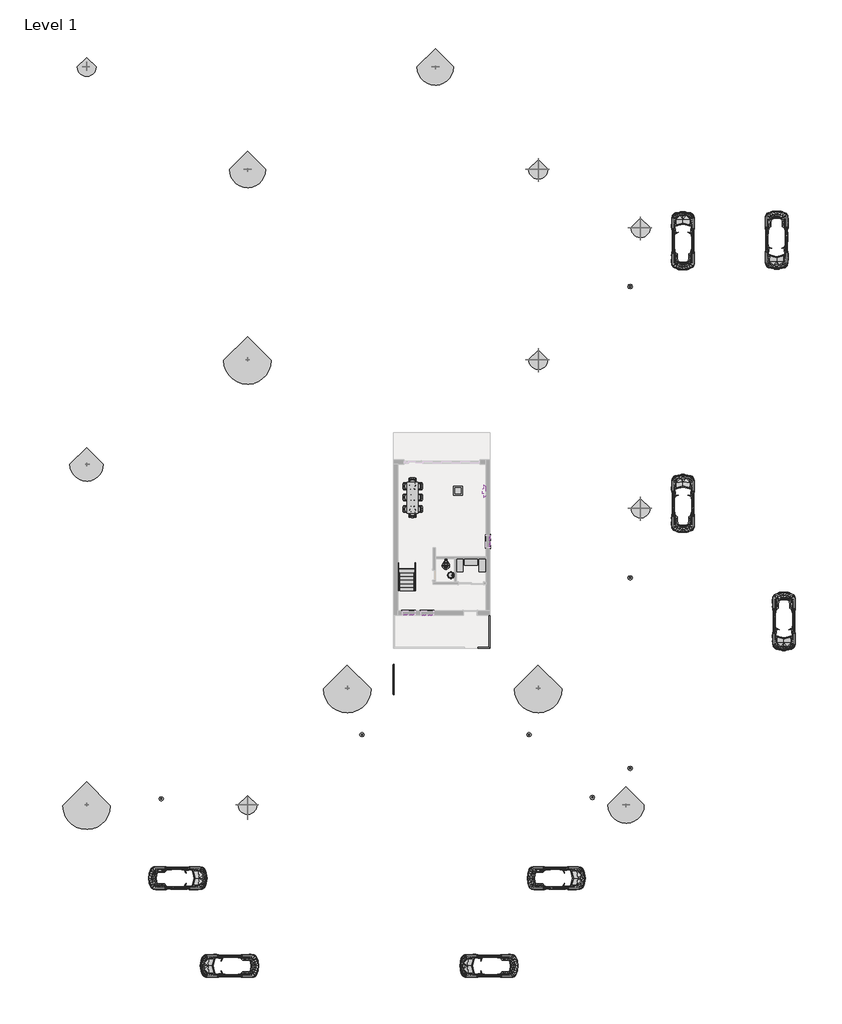
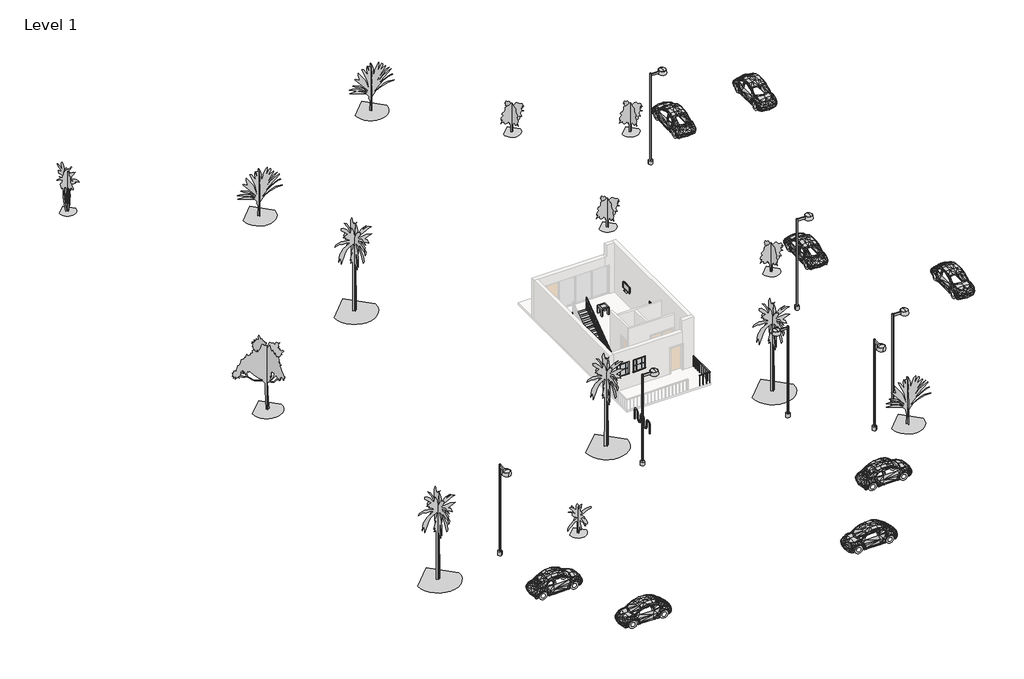
# One storey, part 2 of 2: 21 proxies, 14 furniture elements, 14 geographic elements, 7 light fixtures, 2 flow terminals, 2 members, 2 railings, 1 stair flight.
"""IFC4 building model written with IfcOpenShell, lengths in millimetres."""

from ifc_helpers import new_model, si_unit, frame, origin, origin_with_axes, place, context, project, spatial, polyline, circle_curve, ellipse_curve, outline, extrude, faceted_brep, transform, mapped, element, save
from ifc_brep_helpers import plane_surface, cylinder_surface, advanced_brep
from components import m_bicycle_rack_m_bicycle_rack_69598307, m_muntin_pattern_2x2_m_muntin_pattern_2x2_62480ac4, m_muntin_pattern_2x2_m_muntin_pattern_2x2_4fd78f17, m_rpc_beetle_m_rpc_beetle_aa710b07, m_trim_window_exterior_flat_with_sill_90d3a428, m_trim_window_exterior_flat_with_sill_c06b807c, m_trim_window_interior_flat_picture_frame_6ca9b1f8, m_trim_window_interior_flat_picture_frame_8dc44e6e, m_sink_vanity_round_482_x_482mm_721ec264, m_toilet_commercial_wall_3d_380mm_seat_height_fb359b30, furniture_0810mm_51289c3c, m_furniture_system_storage_cabinet_2_vertical_file_900_x_450_def3fd80, m_seating_auditorium_457_x_610mm_eb3a3c23, m_seating_auditorium_457_x_610mm_4fdbbe14, m_table_coffee_0610_x_0610_x_0610mm_038d1558, m_table_dining_0762_x_2134mm_32ec0f49, m_rpc_tree_tropical_44340318, m_rpc_tree_tropical_0b38fe0e, m_rpc_tree_tropical_cuban_royal_palm_7_5_meters_87faf919, m_rpc_tree_tropical_grass_palm_5_5_meters_0f61173e, m_rpc_tree_tropical_hurricane_palm_3_6_meters_73a83cb7, m_rpc_tree_tropical_japanese_fiber_banana_2_4_meters_2e6d15ad, m_street_light_standard_250w_halogen_277v_204dbcbb, stair_flight_50mm_tread_13mm_riser_6fdf431e

model = new_model("IFC4")

# Units and contexts
model_context = context("Model", 3, world=origin())
ifc_project = project(units=[si_unit("LENGTHUNIT", "METRE", prefix="MILLI")], contexts=[model_context])

# Site, building, storey
site = spatial("IfcSite", under=ifc_project)
building = spatial("IfcBuilding", under=site)
storey = spatial("IfcBuildingStorey", under=building, Name="Level 1", Elevation=0.0)

# Proxies
placement = place(None, origin())
m_bicycle_rack_m_bicycle_rack_shape = m_bicycle_rack_m_bicycle_rack_69598307(model_context)
element("IfcBuildingElementProxy", 1, Name="M_Bicycle Rack : M_Bicycle Rack", ObjectType="M_Bicycle Rack : M_Bicycle Rack", at=placement, inside=storey, context=model_context, shape_type="MappedRepresentation", body=[
    mapped(m_bicycle_rack_m_bicycle_rack_shape, transform((-5369.0317552, -8816.7477501, 0.0), x_axis=(0.0, 1.0, 0.0), y_axis=(-1.0, 0.0, 0.0), z_axis=(0.0, 0.0, 1.0))),
])
m_muntin_pattern_2x2_m_muntin_pattern_2x2_shape = m_muntin_pattern_2x2_m_muntin_pattern_2x2_62480ac4(model_context)
element("IfcBuildingElementProxy", 2, Name="M_Muntin Pattern_2x2 : M_Muntin Pattern_2x2", ObjectType="M_Muntin Pattern_2x2 : M_Muntin Pattern_2x2", at=placement, inside=storey, context=model_context, shape_type="MappedRepresentation", body=[
    mapped(m_muntin_pattern_2x2_m_muntin_pattern_2x2_shape, transform((-4133.1192552, -4407.2227501, 1303.85), x_axis=(-1.0, 0.0, 0.0), y_axis=(0.0, -1.0, 0.0), z_axis=(0.0, 0.0, 1.0))),
])
element("IfcBuildingElementProxy", 3, Name="M_Muntin Pattern_2x2 : M_Muntin Pattern_2x2", ObjectType="M_Muntin Pattern_2x2 : M_Muntin Pattern_2x2", at=placement, inside=storey, context=model_context, shape_type="MappedRepresentation", body=[
    mapped(m_muntin_pattern_2x2_m_muntin_pattern_2x2_shape, transform((-2863.1192552, -4407.2227501, 1303.85), x_axis=(-1.0, 0.0, 0.0), y_axis=(0.0, -1.0, 0.0), z_axis=(0.0, 0.0, 1.0))),
])
element("IfcBuildingElementProxy", 4, Name="M_Muntin Pattern_2x2 : M_Muntin Pattern_2x2", ObjectType="M_Muntin Pattern_2x2 : M_Muntin Pattern_2x2", at=placement, inside=storey, context=model_context, shape_type="MappedRepresentation", body=[
    mapped(m_muntin_pattern_2x2_m_muntin_pattern_2x2_shape, transform((1221.4432448, 819.1647499, 1303.85), x_axis=(0.0, -1.0, 0.0), y_axis=(1.0, 0.0, 0.0), z_axis=(0.0, 0.0, 1.0))),
])
m_muntin_pattern_2x2_m_muntin_pattern_2x2_2_shape = m_muntin_pattern_2x2_m_muntin_pattern_2x2_4fd78f17(model_context)
element("IfcBuildingElementProxy", 5, Name="M_Muntin Pattern_2x2 : M_Muntin Pattern_2x2", ObjectType="M_Muntin Pattern_2x2 : M_Muntin Pattern_2x2", at=placement, inside=storey, context=model_context, shape_type="MappedRepresentation", body=[
    mapped(m_muntin_pattern_2x2_m_muntin_pattern_2x2_2_shape, transform((-4554.9442552, -4407.2227501, 1303.85), x_axis=(1.0, 0.0, 0.0), y_axis=(0.0, 1.0, 0.0), z_axis=(0.0, 0.0, 1.0))),
])
element("IfcBuildingElementProxy", 6, Name="M_Muntin Pattern_2x2 : M_Muntin Pattern_2x2", ObjectType="M_Muntin Pattern_2x2 : M_Muntin Pattern_2x2", at=placement, inside=storey, context=model_context, shape_type="MappedRepresentation", body=[
    mapped(m_muntin_pattern_2x2_m_muntin_pattern_2x2_2_shape, transform((-3284.9442552, -4407.2227501, 1303.85), x_axis=(1.0, 0.0, 0.0), y_axis=(0.0, 1.0, 0.0), z_axis=(0.0, 0.0, 1.0))),
])
element("IfcBuildingElementProxy", 7, Name="M_Muntin Pattern_2x2 : M_Muntin Pattern_2x2", ObjectType="M_Muntin Pattern_2x2 : M_Muntin Pattern_2x2", at=placement, inside=storey, context=model_context, shape_type="MappedRepresentation", body=[
    mapped(m_muntin_pattern_2x2_m_muntin_pattern_2x2_2_shape, transform((1221.4432448, 397.3397499, 1303.85), x_axis=(0.0, 1.0, 0.0), y_axis=(-1.0, 0.0, 0.0), z_axis=(0.0, 0.0, 1.0))),
])
m_rpc_beetle_m_rpc_beetle_shape = m_rpc_beetle_m_rpc_beetle_aa710b07(model_context)
element("IfcBuildingElementProxy", 8, Name="M_RPC Beetle : M_RPC Beetle", ObjectType="M_RPC Beetle : M_RPC Beetle", at=placement, inside=storey, context=model_context, shape_type="MappedRepresentation", body=[
    mapped(m_rpc_beetle_m_rpc_beetle_shape, transform((14420.1682448, 1983.2522499, -152.4), x_axis=(1.0, 0.0, 0.0), y_axis=(0.0, 1.0, 0.0), z_axis=(0.0, 0.0, 1.0))),
])
element("IfcBuildingElementProxy", 9, Name="M_RPC Beetle : M_RPC Beetle", ObjectType="M_RPC Beetle : M_RPC Beetle", at=placement, inside=storey, context=model_context, shape_type="MappedRepresentation", body=[
    mapped(m_rpc_beetle_m_rpc_beetle_shape, transform((21320.1682448, -3616.7477501, -152.4), x_axis=(-1.0, 0.0, 0.0), y_axis=(0.0, -1.0, 0.0), z_axis=(0.0, 0.0, 1.0))),
])
element("IfcBuildingElementProxy", 10, Name="M_RPC Beetle : M_RPC Beetle", ObjectType="M_RPC Beetle : M_RPC Beetle", at=placement, inside=storey, context=model_context, shape_type="MappedRepresentation", body=[
    mapped(m_rpc_beetle_m_rpc_beetle_shape, transform((20820.1682448, 22434.2726811, -152.4), x_axis=(-1.0, 0.0, 0.0), y_axis=(0.0, -1.0, 0.0), z_axis=(0.0, 0.0, 1.0))),
])
element("IfcBuildingElementProxy", 11, Name="M_RPC Beetle : M_RPC Beetle", ObjectType="M_RPC Beetle : M_RPC Beetle", at=placement, inside=storey, context=model_context, shape_type="MappedRepresentation", body=[
    mapped(m_rpc_beetle_m_rpc_beetle_shape, transform((14420.1682448, 19934.2726811, -152.4), x_axis=(1.0, 0.0, 0.0), y_axis=(0.0, 1.0, 0.0), z_axis=(0.0, 0.0, 1.0))),
])
element("IfcBuildingElementProxy", 12, Name="M_RPC Beetle : M_RPC Beetle", ObjectType="M_RPC Beetle : M_RPC Beetle", at=placement, inside=storey, context=model_context, shape_type="MappedRepresentation", body=[
    mapped(m_rpc_beetle_m_rpc_beetle_shape, transform((4520.1682448, -22389.3361723, -152.4), x_axis=(0.0, -1.0, 0.0), y_axis=(1.0, 0.0, 0.0), z_axis=(0.0, 0.0, 1.0))),
])
element("IfcBuildingElementProxy", 13, Name="M_RPC Beetle : M_RPC Beetle", ObjectType="M_RPC Beetle : M_RPC Beetle", at=placement, inside=storey, context=model_context, shape_type="MappedRepresentation", body=[
    mapped(m_rpc_beetle_m_rpc_beetle_shape, transform((2380.1682448, -28389.3361723, -152.4), x_axis=(0.0, 1.0, 0.0), y_axis=(-1.0, 0.0, 0.0), z_axis=(0.0, 0.0, 1.0))),
])
element("IfcBuildingElementProxy", 14, Name="M_RPC Beetle : M_RPC Beetle", ObjectType="M_RPC Beetle : M_RPC Beetle", at=placement, inside=storey, context=model_context, shape_type="MappedRepresentation", body=[
    mapped(m_rpc_beetle_m_rpc_beetle_shape, transform((-15353.4317552, -28389.3361723, -152.4), x_axis=(0.0, 1.0, 0.0), y_axis=(-1.0, 0.0, 0.0), z_axis=(0.0, 0.0, 1.0))),
])
element("IfcBuildingElementProxy", 15, Name="M_RPC Beetle : M_RPC Beetle", ObjectType="M_RPC Beetle : M_RPC Beetle", at=placement, inside=storey, context=model_context, shape_type="MappedRepresentation", body=[
    mapped(m_rpc_beetle_m_rpc_beetle_shape, transform((-21353.4317552, -22389.3361723, -152.4), x_axis=(0.0, -1.0, 0.0), y_axis=(1.0, 0.0, 0.0), z_axis=(0.0, 0.0, 1.0))),
])
m_trim_window_exterior_flat_with_sill_shape = m_trim_window_exterior_flat_with_sill_90d3a428(model_context)
element("IfcBuildingElementProxy", 16, Name="M_Trim-Window-Exterior-Flat : with Sill", ObjectType="M_Trim-Window-Exterior-Flat : with Sill", at=placement, inside=storey, context=model_context, shape_type="MappedRepresentation", body=[
    mapped(m_trim_window_exterior_flat_with_sill_shape, transform((-4344.0317552, -4416.7477501, 2134.0), x_axis=(1.0, 0.0, 0.0), y_axis=(0.0, 0.0, 1.0), z_axis=(0.0, -1.0, 0.0))),
])
element("IfcBuildingElementProxy", 17, Name="M_Trim-Window-Exterior-Flat : with Sill", ObjectType="M_Trim-Window-Exterior-Flat : with Sill", at=placement, inside=storey, context=model_context, shape_type="MappedRepresentation", body=[
    mapped(m_trim_window_exterior_flat_with_sill_shape, transform((-3074.0317552, -4416.7477501, 2134.0), x_axis=(1.0, 0.0, 0.0), y_axis=(0.0, 0.0, 1.0), z_axis=(0.0, -1.0, 0.0))),
])
m_trim_window_exterior_flat_with_sill_2_shape = m_trim_window_exterior_flat_with_sill_c06b807c(model_context)
element("IfcBuildingElementProxy", 18, Name="M_Trim-Window-Exterior-Flat : with Sill", ObjectType="M_Trim-Window-Exterior-Flat : with Sill", at=placement, inside=storey, context=model_context, shape_type="MappedRepresentation", body=[
    mapped(m_trim_window_exterior_flat_with_sill_2_shape, transform((1230.9682448, 608.2522499, 2134.0), x_axis=(0.0, -1.0, 0.0), y_axis=(0.0, 0.0, -1.0), z_axis=(1.0, 0.0, 0.0))),
])
m_trim_window_interior_flat_picture_frame_shape = m_trim_window_interior_flat_picture_frame_6ca9b1f8(model_context)
element("IfcBuildingElementProxy", 19, Name="M_Trim-Window-Interior-Flat : Picture Frame", ObjectType="M_Trim-Window-Interior-Flat : Picture Frame", at=placement, inside=storey, context=model_context, shape_type="MappedRepresentation", body=[
    mapped(m_trim_window_interior_flat_picture_frame_shape, transform((-4344.0317552, -4116.7477501, 2134.0), x_axis=(-1.0, 0.0, 0.0), y_axis=(0.0, 0.0, 1.0), z_axis=(0.0, 1.0, 0.0))),
])
element("IfcBuildingElementProxy", 20, Name="M_Trim-Window-Interior-Flat : Picture Frame", ObjectType="M_Trim-Window-Interior-Flat : Picture Frame", at=placement, inside=storey, context=model_context, shape_type="MappedRepresentation", body=[
    mapped(m_trim_window_interior_flat_picture_frame_shape, transform((-3074.0317552, -4116.7477501, 2134.0), x_axis=(-1.0, 0.0, 0.0), y_axis=(0.0, 0.0, 1.0), z_axis=(0.0, 1.0, 0.0))),
])
m_trim_window_interior_flat_picture_frame_2_shape = m_trim_window_interior_flat_picture_frame_8dc44e6e(model_context)
element("IfcBuildingElementProxy", 21, Name="M_Trim-Window-Interior-Flat : Picture Frame", ObjectType="M_Trim-Window-Interior-Flat : Picture Frame", at=placement, inside=storey, context=model_context, shape_type="MappedRepresentation", body=[
    mapped(m_trim_window_interior_flat_picture_frame_2_shape, transform((930.9682448, 608.2522499, 2134.0), x_axis=(0.0, 1.0, 0.0), y_axis=(0.0, 0.0, -1.0), z_axis=(-1.0, 0.0, 0.0))),
])

# Flow terminals
m_sink_vanity_round_482_x_482mm_shape = m_sink_vanity_round_482_x_482mm_721ec264(model_context)
element("IfcFlowTerminal", 22, ObjectType="M_Sink Vanity-Round : 482 x 482mm", at=placement, inside=storey, context=model_context, shape_type="MappedRepresentation", body=[
    mapped(m_sink_vanity_round_482_x_482mm_shape, transform((-1544.5577535, -1590.0960096, 0.0), x_axis=(0.0, -1.0, 0.0), y_axis=(1.0, 0.0, 0.0), z_axis=(0.0, 0.0, 1.0))),
])
m_toilet_commercial_wall_3d_380mm_seat_height_shape = m_toilet_commercial_wall_3d_380mm_seat_height_fb359b30(model_context)
element("IfcFlowTerminal", 23, ObjectType="M_Toilet-Commercial-Wall-3D : 380mm Seat Height", at=placement, inside=storey, context=model_context, shape_type="MappedRepresentation", body=[
    mapped(m_toilet_commercial_wall_3d_380mm_seat_height_shape, transform((-1388.1286014, -491.7477501, 0.0), x_axis=(-1.0, 0.0, 0.0), y_axis=(0.0, -1.0, 0.0), z_axis=(0.0, 0.0, 1.0))),
])

# Furniture
furniture_0810mm_shape = furniture_0810mm_51289c3c(model_context)
element("IfcFurniture", 24, ObjectType="0810mm", at=placement, inside=storey, context=model_context, shape_type="MappedRepresentation", body=[
    mapped(furniture_0810mm_shape, transform((866.2308395, 4039.3077357, 1219.2), x_axis=(0.0, -1.0, 0.0), y_axis=(1.0, 0.0, 0.0), z_axis=(0.0, 0.0, 1.0))),
])
m_furniture_system_storage_cabinet_2_vertical_file_900_x_450_shape = m_furniture_system_storage_cabinet_2_vertical_file_900_x_450_def3fd80(model_context)
element("IfcFurniture", 25, ObjectType="M_Furniture_System-Storage-Cabinet-2_Vertical_File : 900 x 450 x 650mm", at=placement, inside=storey, context=model_context, shape_type="MappedRepresentation", body=[
    mapped(m_furniture_system_storage_cabinet_2_vertical_file_900_x_450_shape, transform((-619.0317552, -1016.7477501, 0.0), x_axis=(0.0, 1.0, 0.0), y_axis=(-1.0, 0.0, 0.0), z_axis=(0.0, 0.0, 1.0))),
])
element("IfcFurniture", 26, ObjectType="M_Furniture_System-Storage-Cabinet-2_Vertical_File : 900 x 450 x 650mm", at=placement, inside=storey, context=model_context, shape_type="MappedRepresentation", body=[
    mapped(m_furniture_system_storage_cabinet_2_vertical_file_900_x_450_shape, transform((480.9682448, -1016.7477501, 0.0), x_axis=(0.0, -1.0, 0.0), y_axis=(1.0, 0.0, 0.0), z_axis=(0.0, 0.0, 1.0))),
])
element("IfcFurniture", 27, ObjectType="M_Furniture_System-Storage-Cabinet-2_Vertical_File : 900 x 450 x 650mm", at=placement, inside=storey, context=model_context, shape_type="MappedRepresentation", body=[
    mapped(m_furniture_system_storage_cabinet_2_vertical_file_900_x_450_shape, transform((-69.0317552, -1016.7477501, 0.0), x_axis=(1.0, 0.0, 0.0), y_axis=(0.0, 1.0, 0.0), z_axis=(0.0, 0.0, 1.0))),
])
m_seating_auditorium_457_x_610mm_shape = m_seating_auditorium_457_x_610mm_eb3a3c23(model_context)
element("IfcFurniture", 28, ObjectType="M_Seating-Auditorium : 457 x 610mm", at=placement, inside=storey, context=model_context, shape_type="MappedRepresentation", body=[
    mapped(m_seating_auditorium_457_x_610mm_shape, transform((-4639.907165, 4542.5801187, 0.0), x_axis=(0.0, -1.0, 0.0), y_axis=(1.0, 0.0, 0.0), z_axis=(0.0, 0.0, 1.0))),
])
element("IfcFurniture", 29, ObjectType="M_Seating-Auditorium : 457 x 610mm", at=placement, inside=storey, context=model_context, shape_type="MappedRepresentation", body=[
    mapped(m_seating_auditorium_457_x_610mm_shape, transform((-3498.1563454, 4221.124381, 0.0), x_axis=(0.0, 1.0, 0.0), y_axis=(-1.0, 0.0, 0.0), z_axis=(0.0, 0.0, 1.0))),
])
element("IfcFurniture", 30, ObjectType="M_Seating-Auditorium : 457 x 610mm", at=placement, inside=storey, context=model_context, shape_type="MappedRepresentation", body=[
    mapped(m_seating_auditorium_457_x_610mm_shape, transform((-3908.3038863, 4860.1276597, 0.0), x_axis=(-1.0, 0.0, 0.0), y_axis=(0.0, -1.0, 0.0), z_axis=(0.0, 0.0, 1.0))),
])
element("IfcFurniture", 31, ObjectType="M_Seating-Auditorium : 457 x 610mm", at=placement, inside=storey, context=model_context, shape_type="MappedRepresentation", body=[
    mapped(m_seating_auditorium_457_x_610mm_shape, transform((-4229.759624, 2346.37684, 0.0), x_axis=(1.0, 0.0, 0.0), y_axis=(0.0, 1.0, 0.0), z_axis=(0.0, 0.0, 1.0))),
])
m_seating_auditorium_457_x_610mm_2_shape = m_seating_auditorium_457_x_610mm_4fdbbe14(model_context)
element("IfcFurniture", 32, ObjectType="M_Seating-Auditorium : 457 x 610mm", at=placement, inside=storey, context=model_context, shape_type="MappedRepresentation", body=[
    mapped(m_seating_auditorium_457_x_610mm_2_shape, transform((-4639.907165, 2663.924381, 0.0), x_axis=(0.0, 1.0, 0.0), y_axis=(-1.0, 0.0, 0.0), z_axis=(0.0, 0.0, 1.0))),
])
element("IfcFurniture", 33, ObjectType="M_Seating-Auditorium : 457 x 610mm", at=placement, inside=storey, context=model_context, shape_type="MappedRepresentation", body=[
    mapped(m_seating_auditorium_457_x_610mm_2_shape, transform((-3498.1563454, 2985.3801187, 0.0), x_axis=(0.0, -1.0, 0.0), y_axis=(1.0, 0.0, 0.0), z_axis=(0.0, 0.0, 1.0))),
])
element("IfcFurniture", 34, ObjectType="M_Seating-Auditorium : 457 x 610mm", at=placement, inside=storey, context=model_context, shape_type="MappedRepresentation", body=[
    mapped(m_seating_auditorium_457_x_610mm_2_shape, transform((-4639.907165, 3463.924381, 0.0), x_axis=(0.0, 1.0, 0.0), y_axis=(-1.0, 0.0, 0.0), z_axis=(0.0, 0.0, 1.0))),
])
element("IfcFurniture", 35, ObjectType="M_Seating-Auditorium : 457 x 610mm", at=placement, inside=storey, context=model_context, shape_type="MappedRepresentation", body=[
    mapped(m_seating_auditorium_457_x_610mm_2_shape, transform((-3498.1563454, 3785.3801187, 0.0), x_axis=(0.0, -1.0, 0.0), y_axis=(1.0, 0.0, 0.0), z_axis=(0.0, 0.0, 1.0))),
])
m_table_coffee_0610_x_0610_x_0610mm_shape = m_table_coffee_0610_x_0610_x_0610mm_038d1558(model_context)
element("IfcFurniture", 36, ObjectType="M_Table-Coffee : 0610 x 0610 x 0610mm", at=placement, inside=storey, context=model_context, shape_type="MappedRepresentation", body=[
    mapped(m_table_coffee_0610_x_0610_x_0610mm_shape, transform((-997.2975219, 3978.0411721, 0.0), x_axis=(1.0, 0.0, 0.0), y_axis=(0.0, 1.0, 0.0), z_axis=(0.0, 0.0, 1.0))),
])
m_table_dining_0762_x_2134mm_shape = m_table_dining_0762_x_2134mm_32ec0f49(model_context)
element("IfcFurniture", 37, ObjectType="M_Table-Dining : 0762 x 2134mm", at=placement, inside=storey, context=model_context, shape_type="MappedRepresentation", body=[
    mapped(m_table_dining_0762_x_2134mm_shape, transform((-3973.8206774, 3584.9864832, 0.0), x_axis=(0.0, 1.0, 0.0), y_axis=(-1.0, 0.0, 0.0), z_axis=(0.0, 0.0, 1.0))),
])

# Geographic elements
m_rpc_tree_tropical_shape = m_rpc_tree_tropical_44340318(model_context)
element("IfcGeographicElement", 38, ObjectType="M_RPC Tree - Tropical", at=placement, inside=storey, context=model_context, shape_type="MappedRepresentation", body=[
    mapped(m_rpc_tree_tropical_shape, transform((10519.9715737, -17389.3361723, -152.4), x_axis=(1.0, 0.0, 0.0), y_axis=(0.0, 1.0, 0.0), z_axis=(0.0, 0.0, 1.0))),
])
element("IfcGeographicElement", 39, ObjectType="M_RPC Tree - Tropical", at=placement, inside=storey, context=model_context, shape_type="MappedRepresentation", body=[
    mapped(m_rpc_tree_tropical_shape, transform((-2519.2284263, 33034.2726811, -152.4), x_axis=(1.0, 0.0, 0.0), y_axis=(0.0, 1.0, 0.0), z_axis=(0.0, 0.0, 1.0))),
])
element("IfcGeographicElement", 40, ObjectType="M_RPC Tree - Tropical", at=placement, inside=storey, context=model_context, shape_type="MappedRepresentation", body=[
    mapped(m_rpc_tree_tropical_shape, transform((-15353.6284263, 26034.2726811, -152.4), x_axis=(1.0, 0.0, 0.0), y_axis=(0.0, 1.0, 0.0), z_axis=(0.0, 0.0, 1.0))),
])
m_rpc_tree_tropical_2_shape = m_rpc_tree_tropical_0b38fe0e(model_context)
element("IfcGeographicElement", 41, ObjectType="M_RPC Tree - Tropical", at=placement, inside=storey, context=model_context, shape_type="MappedRepresentation", body=[
    mapped(m_rpc_tree_tropical_2_shape, transform((11519.9715737, 2883.2522499, -152.4), x_axis=(1.0, 0.0, 0.0), y_axis=(0.0, 1.0, 0.0), z_axis=(0.0, 0.0, 1.0))),
])
element("IfcGeographicElement", 42, ObjectType="M_RPC Tree - Tropical", at=placement, inside=storey, context=model_context, shape_type="MappedRepresentation", body=[
    mapped(m_rpc_tree_tropical_2_shape, transform((11519.9715737, 22034.2726811, -152.4), x_axis=(1.0, 0.0, 0.0), y_axis=(0.0, 1.0, 0.0), z_axis=(0.0, 0.0, 1.0))),
])
element("IfcGeographicElement", 43, ObjectType="M_RPC Tree - Tropical", at=placement, inside=storey, context=model_context, shape_type="MappedRepresentation", body=[
    mapped(m_rpc_tree_tropical_2_shape, transform((4519.9715737, 26034.2726811, -152.4), x_axis=(1.0, 0.0, 0.0), y_axis=(0.0, 1.0, 0.0), z_axis=(0.0, 0.0, 1.0))),
])
element("IfcGeographicElement", 44, ObjectType="M_RPC Tree - Tropical", at=placement, inside=storey, context=model_context, shape_type="MappedRepresentation", body=[
    mapped(m_rpc_tree_tropical_2_shape, transform((4519.9715737, 13034.2726811, -152.4), x_axis=(1.0, 0.0, 0.0), y_axis=(0.0, 1.0, 0.0), z_axis=(0.0, 0.0, 1.0))),
])
m_rpc_tree_tropical_cuban_royal_palm_7_5_meters_shape = m_rpc_tree_tropical_cuban_royal_palm_7_5_meters_87faf919(model_context)
element("IfcGeographicElement", 45, ObjectType="M_RPC Tree - Tropical : Cuban Royal Palm - 7.5 Meters", at=placement, inside=storey, context=model_context, shape_type="MappedRepresentation", body=[
    mapped(m_rpc_tree_tropical_cuban_royal_palm_7_5_meters_shape, transform((-8529.2284263, -9416.7477501, -152.4), x_axis=(1.0, 0.0, 0.0), y_axis=(0.0, 1.0, 0.0), z_axis=(0.0, 0.0, 1.0))),
])
element("IfcGeographicElement", 46, ObjectType="M_RPC Tree - Tropical : Cuban Royal Palm - 7.5 Meters", at=placement, inside=storey, context=model_context, shape_type="MappedRepresentation", body=[
    mapped(m_rpc_tree_tropical_cuban_royal_palm_7_5_meters_shape, transform((4519.9715737, -9416.7477501, -152.4), x_axis=(1.0, 0.0, 0.0), y_axis=(0.0, 1.0, 0.0), z_axis=(0.0, 0.0, 1.0))),
])
element("IfcGeographicElement", 47, ObjectType="M_RPC Tree - Tropical : Cuban Royal Palm - 7.5 Meters", at=placement, inside=storey, context=model_context, shape_type="MappedRepresentation", body=[
    mapped(m_rpc_tree_tropical_cuban_royal_palm_7_5_meters_shape, transform((-26353.6284263, -17389.3361723, -152.4), x_axis=(1.0, 0.0, 0.0), y_axis=(0.0, 1.0, 0.0), z_axis=(0.0, 0.0, 1.0))),
])
element("IfcGeographicElement", 48, ObjectType="M_RPC Tree - Tropical : Cuban Royal Palm - 7.5 Meters", at=placement, inside=storey, context=model_context, shape_type="MappedRepresentation", body=[
    mapped(m_rpc_tree_tropical_cuban_royal_palm_7_5_meters_shape, transform((-15353.6284263, 13034.2726811, -152.4), x_axis=(1.0, 0.0, 0.0), y_axis=(0.0, 1.0, 0.0), z_axis=(0.0, 0.0, 1.0))),
])
m_rpc_tree_tropical_grass_palm_5_5_meters_shape = m_rpc_tree_tropical_grass_palm_5_5_meters_0f61173e(model_context)
element("IfcGeographicElement", 49, ObjectType="M_RPC Tree - Tropical : Grass Palm - 5.5 Meters", at=placement, inside=storey, context=model_context, shape_type="MappedRepresentation", body=[
    mapped(m_rpc_tree_tropical_grass_palm_5_5_meters_shape, transform((-26353.6284263, 5883.2522499, -152.4), x_axis=(1.0, 0.0, 0.0), y_axis=(0.0, 1.0, 0.0), z_axis=(0.0, 0.0, 1.0))),
])
m_rpc_tree_tropical_hurricane_palm_3_6_meters_shape = m_rpc_tree_tropical_hurricane_palm_3_6_meters_73a83cb7(model_context)
element("IfcGeographicElement", 50, ObjectType="M_RPC Tree - Tropical : Hurricane Palm - 3.6 Meters", at=placement, inside=storey, context=model_context, shape_type="MappedRepresentation", body=[
    mapped(m_rpc_tree_tropical_hurricane_palm_3_6_meters_shape, transform((-26353.6284263, 33034.2726811, -152.4), x_axis=(1.0, 0.0, 0.0), y_axis=(0.0, 1.0, 0.0), z_axis=(0.0, 0.0, 1.0))),
])
m_rpc_tree_tropical_japanese_fiber_banana_2_4_meters_shape = m_rpc_tree_tropical_japanese_fiber_banana_2_4_meters_2e6d15ad(model_context)
element("IfcGeographicElement", 51, ObjectType="M_RPC Tree - Tropical : Japanese Fiber Banana - 2.4 Meters", at=placement, inside=storey, context=model_context, shape_type="MappedRepresentation", body=[
    mapped(m_rpc_tree_tropical_japanese_fiber_banana_2_4_meters_shape, transform((-15353.6284263, -17389.3361723, -152.4), x_axis=(1.0, 0.0, 0.0), y_axis=(0.0, 1.0, 0.0), z_axis=(0.0, 0.0, 1.0))),
])

# Light fixtures
m_street_light_standard_250w_halogen_277v_shape = m_street_light_standard_250w_halogen_277v_204dbcbb(model_context)
element("IfcLightFixture", 52, ObjectType="M_Street Light - Standard", at=placement, inside=storey, context=model_context, shape_type="MappedRepresentation", body=[
    mapped(m_street_light_standard_250w_halogen_277v_shape, transform((-7527.8317552, -12589.3361723, -152.4), x_axis=(-1.0, 0.0, 0.0), y_axis=(0.0, -1.0, 0.0), z_axis=(0.0, 0.0, 1.0))),
])
element("IfcLightFixture", 53, ObjectType="M_Street Light - Standard : 250W Halogen - 277V", at=placement, inside=storey, context=model_context, shape_type="MappedRepresentation", body=[
    mapped(m_street_light_standard_250w_halogen_277v_shape, transform((3894.5682448, -12589.3361723, -152.4), x_axis=(1.0, 0.0, 0.0), y_axis=(0.0, 1.0, 0.0), z_axis=(0.0, 0.0, 1.0))),
])
element("IfcLightFixture", 54, ObjectType="M_Street Light - Standard : 400W Halogen - 120V", at=placement, inside=storey, context=model_context, shape_type="MappedRepresentation", body=[
    mapped(m_street_light_standard_250w_halogen_277v_shape, transform((8220.1682448, -16874.9361723, -152.4), x_axis=(0.0, 1.0, 0.0), y_axis=(-1.0, 0.0, 0.0), z_axis=(0.0, 0.0, 1.0))),
])
element("IfcLightFixture", 55, ObjectType="M_Street Light - Standard : 400W Halogen - 120V", at=placement, inside=storey, context=model_context, shape_type="MappedRepresentation", body=[
    mapped(m_street_light_standard_250w_halogen_277v_shape, transform((10805.7682448, -14889.3361723, -152.4), x_axis=(-1.0, 0.0, 0.0), y_axis=(0.0, -1.0, 0.0), z_axis=(0.0, 0.0, 1.0))),
])
element("IfcLightFixture", 56, ObjectType="M_Street Light - Standard : 400W Halogen - 120V", at=placement, inside=storey, context=model_context, shape_type="MappedRepresentation", body=[
    mapped(m_street_light_standard_250w_halogen_277v_shape, transform((10805.7682448, -1866.7477501, -152.4), x_axis=(-1.0, 0.0, 0.0), y_axis=(0.0, -1.0, 0.0), z_axis=(0.0, 0.0, 1.0))),
])
element("IfcLightFixture", 57, ObjectType="M_Street Light - Standard : 400W Halogen - 120V", at=placement, inside=storey, context=model_context, shape_type="MappedRepresentation", body=[
    mapped(m_street_light_standard_250w_halogen_277v_shape, transform((10805.7682448, 18034.2726811, -152.4), x_axis=(-1.0, 0.0, 0.0), y_axis=(0.0, -1.0, 0.0), z_axis=(0.0, 0.0, 1.0))),
])
element("IfcLightFixture", 58, ObjectType="M_Street Light - Standard : 400W Halogen - 120V", at=placement, inside=storey, context=model_context, shape_type="MappedRepresentation", body=[
    mapped(m_street_light_standard_250w_halogen_277v_shape, transform((-21253.4317552, -16974.9361723, -152.4), x_axis=(0.0, 1.0, 0.0), y_axis=(-1.0, 0.0, 0.0), z_axis=(0.0, 0.0, 1.0))),
])

# Members
element("IfcMember", 59, ObjectType="Stringer - 50mm Width", at=placement, inside=storey, context=model_context, shape_type="SweptSolid", body=[
    extrude(outline(polyline([(-2766.7477501, 0.0), (-2766.7477501, 253.5299646), (1233.2522499, 3265.2946705), (1233.2522499, 2764.5879036), (-2438.4660596, 0.0), (-2766.7477501, 0.0)])), frame((-5069.0317552, 0.0, 0.0), z_axis=(1.0, 0.0, 0.0), x_axis=(0.0, 1.0, 0.0)), (0.0, 0.0, 1.0), 50.0),
])
element("IfcMember", 60, ObjectType="Stringer - 50mm Width", at=placement, inside=storey, context=model_context, shape_type="SweptSolid", body=[
    extrude(outline(polyline([(-2766.7477501, 0.0), (-2766.7477501, 253.5299646), (1233.2522499, 3265.2946705), (1233.2522499, 2764.5879036), (-2438.4660596, 0.0), (-2766.7477501, 0.0)])), frame((-3919.0317552, 0.0, 0.0), z_axis=(1.0, 0.0, 0.0), x_axis=(0.0, 1.0, 0.0)), (0.0, 0.0, 1.0), 50.0),
])

# Railings
element("IfcRailing", 61, ObjectType="900mm Pipe", at=placement, inside=storey, context=model_context, shape_type="AdvancedBrep", body=[
    advanced_brep(
    [(-3924.4317552, -2766.7477501, 1063.1999558), (-3964.4317552, -2766.7477501, 1063.1999558), (-3924.4317552, 1233.2522499, 4074.9646617), (-3964.4317552, 1233.2522499, 4074.9646617)],
    [
        (0, 1, ellipse_curve(frame((-3944.4317552, -2766.7477501, 1063.1999558), z_axis=(0.0, -1.0, 0.0), x_axis=(0.0, 0.0, -1.0)), 25.0353383, 20.0)),
        (1, 0, ellipse_curve(frame((-3944.4317552, -2766.7477501, 1063.1999558), z_axis=(0.0, -1.0, 0.0), x_axis=(0.0, 0.0, -1.0)), 25.0353383, 20.0)),
        (2, 3, ellipse_curve(frame((-3944.4317552, 1233.2522499, 4074.9646617), z_axis=(0.0, 1.0, 0.0), x_axis=(0.0, 0.0, -1.0)), 25.0353383, 20.0)),
        (3, 2, ellipse_curve(frame((-3944.4317552, 1233.2522499, 4074.9646617), z_axis=(0.0, 1.0, 0.0), x_axis=(0.0, 0.0, -1.0)), 25.0353383, 20.0)),
        (0, 2),
        (3, 1),
    ],
    [
        plane_surface(frame((-3944.4317552, -2766.7477501, 1088.2352941), z_axis=(0.0, -1.0, 0.0), x_axis=(0.0, 0.0, 1.0))),
        plane_surface(frame((-3944.4317552, 1233.2522499, 4100.0), z_axis=(0.0, 1.0, 0.0), x_axis=(0.0, 0.0, 1.0))),
        cylinder_surface(frame((-3944.4317552, -2754.7176962, 1072.2578787), z_axis=(0.0, -0.7988707691396074, -0.6015026967639399), x_axis=(-1.0, 0.0, 0.0)), 20.0),
    ],
    [
        (0, [[1, 2]]),
        (1, [[3, 4]]),
        (2, [[-1, 5, -4, 6]]),
        (2, [[-2, -6, -3, -5]]),
    ],
),
    advanced_brep(
    [(-3959.4317552, -2766.7477501, 869.4587904), (-3929.4317552, -2766.7477501, 869.4587904), (-3959.4317552, 1233.2522499, 3881.2234962), (-3929.4317552, 1233.2522499, 3881.2234962)],
    [
        (0, 1, ellipse_curve(frame((-3944.4317552, -2766.7477501, 869.4587904), z_axis=(0.0, -1.0, 0.0), x_axis=(0.0, 0.0, -1.0)), 18.7765038, 15.0)),
        (1, 0, ellipse_curve(frame((-3944.4317552, -2766.7477501, 869.4587904), z_axis=(0.0, -1.0, 0.0), x_axis=(0.0, 0.0, -1.0)), 18.7765038, 15.0)),
        (2, 3, ellipse_curve(frame((-3944.4317552, 1233.2522499, 3881.2234962), z_axis=(0.0, 1.0, 0.0), x_axis=(0.0, 0.0, -1.0)), 18.7765038, 15.0)),
        (3, 2, ellipse_curve(frame((-3944.4317552, 1233.2522499, 3881.2234962), z_axis=(0.0, 1.0, 0.0), x_axis=(0.0, 0.0, -1.0)), 18.7765038, 15.0)),
        (0, 2),
        (3, 1),
    ],
    [
        plane_surface(frame((-3944.4317552, -2766.7477501, 888.2352941), z_axis=(0.0, -1.0, 0.0), x_axis=(0.0, 0.0, 1.0))),
        plane_surface(frame((-3944.4317552, 1233.2522499, 3900.0), z_axis=(0.0, 1.0, 0.0), x_axis=(0.0, 0.0, 1.0))),
        cylinder_surface(frame((-3944.4317552, -2757.7252097, 876.2522326), z_axis=(0.0, -0.7988707691396074, -0.6015026967639399), x_axis=(1.0, 0.0, 0.0)), 15.0),
    ],
    [
        (0, [[1, 2]]),
        (1, [[3, 4]]),
        (2, [[-1, 5, -4, 6]]),
        (2, [[-2, -6, -3, -5]]),
    ],
),
    advanced_brep(
    [(-3959.4317552, -2766.7477501, 669.4587904), (-3929.4317552, -2766.7477501, 669.4587904), (-3959.4317552, 1233.2522499, 3681.2234962), (-3929.4317552, 1233.2522499, 3681.2234962)],
    [
        (0, 1, ellipse_curve(frame((-3944.4317552, -2766.7477501, 669.4587904), z_axis=(0.0, -1.0, 0.0), x_axis=(0.0, 0.0, -1.0)), 18.7765038, 15.0)),
        (1, 0, ellipse_curve(frame((-3944.4317552, -2766.7477501, 669.4587904), z_axis=(0.0, -1.0, 0.0), x_axis=(0.0, 0.0, -1.0)), 18.7765038, 15.0)),
        (2, 3, ellipse_curve(frame((-3944.4317552, 1233.2522499, 3681.2234962), z_axis=(0.0, 1.0, 0.0), x_axis=(0.0, 0.0, -1.0)), 18.7765038, 15.0)),
        (3, 2, ellipse_curve(frame((-3944.4317552, 1233.2522499, 3681.2234962), z_axis=(0.0, 1.0, 0.0), x_axis=(0.0, 0.0, -1.0)), 18.7765038, 15.0)),
        (0, 2),
        (3, 1),
    ],
    [
        plane_surface(frame((-3944.4317552, -2766.7477501, 688.2352941), z_axis=(0.0, -1.0, 0.0), x_axis=(0.0, 0.0, 1.0))),
        plane_surface(frame((-3944.4317552, 1233.2522499, 3700.0), z_axis=(0.0, 1.0, 0.0), x_axis=(0.0, 0.0, 1.0))),
        cylinder_surface(frame((-3944.4317552, -2757.7252097, 676.2522326), z_axis=(0.0, -0.7988707691396074, -0.6015026967639399), x_axis=(1.0, 0.0, 0.0)), 15.0),
    ],
    [
        (0, [[1, 2]]),
        (1, [[3, 4]]),
        (2, [[-1, 5, -4, 6]]),
        (2, [[-2, -6, -3, -5]]),
    ],
),
    advanced_brep(
    [(-3959.4317552, -2766.7477501, 469.4587904), (-3929.4317552, -2766.7477501, 469.4587904), (-3959.4317552, 1233.2522499, 3481.2234962), (-3929.4317552, 1233.2522499, 3481.2234962)],
    [
        (0, 1, ellipse_curve(frame((-3944.4317552, -2766.7477501, 469.4587904), z_axis=(0.0, -1.0, 0.0), x_axis=(0.0, 0.0, -1.0)), 18.7765038, 15.0)),
        (1, 0, ellipse_curve(frame((-3944.4317552, -2766.7477501, 469.4587904), z_axis=(0.0, -1.0, 0.0), x_axis=(0.0, 0.0, -1.0)), 18.7765038, 15.0)),
        (2, 3, ellipse_curve(frame((-3944.4317552, 1233.2522499, 3481.2234962), z_axis=(0.0, 1.0, 0.0), x_axis=(0.0, 0.0, -1.0)), 18.7765038, 15.0)),
        (3, 2, ellipse_curve(frame((-3944.4317552, 1233.2522499, 3481.2234962), z_axis=(0.0, 1.0, 0.0), x_axis=(0.0, 0.0, -1.0)), 18.7765038, 15.0)),
        (0, 2),
        (3, 1),
    ],
    [
        plane_surface(frame((-3944.4317552, -2766.7477501, 488.2352941), z_axis=(0.0, -1.0, 0.0), x_axis=(0.0, 0.0, 1.0))),
        plane_surface(frame((-3944.4317552, 1233.2522499, 3500.0), z_axis=(0.0, 1.0, 0.0), x_axis=(0.0, 0.0, 1.0))),
        cylinder_surface(frame((-3944.4317552, -2757.7252097, 476.2522326), z_axis=(0.0, -0.7988707691396074, -0.6015026967639399), x_axis=(1.0, 0.0, 0.0)), 15.0),
    ],
    [
        (0, [[1, 2]]),
        (1, [[3, 4]]),
        (2, [[-1, 5, -4, 6]]),
        (2, [[-2, -6, -3, -5]]),
    ],
),
    advanced_brep(
    [(-3959.4317552, -2766.7477501, 269.4587904), (-3929.4317552, -2766.7477501, 269.4587904), (-3959.4317552, 1233.2522499, 3281.2234962), (-3929.4317552, 1233.2522499, 3281.2234962)],
    [
        (0, 1, ellipse_curve(frame((-3944.4317552, -2766.7477501, 269.4587904), z_axis=(0.0, -1.0, 0.0), x_axis=(0.0, 0.0, -1.0)), 18.7765038, 15.0)),
        (1, 0, ellipse_curve(frame((-3944.4317552, -2766.7477501, 269.4587904), z_axis=(0.0, -1.0, 0.0), x_axis=(0.0, 0.0, -1.0)), 18.7765038, 15.0)),
        (2, 3, ellipse_curve(frame((-3944.4317552, 1233.2522499, 3281.2234962), z_axis=(0.0, 1.0, 0.0), x_axis=(0.0, 0.0, -1.0)), 18.7765038, 15.0)),
        (3, 2, ellipse_curve(frame((-3944.4317552, 1233.2522499, 3281.2234962), z_axis=(0.0, 1.0, 0.0), x_axis=(0.0, 0.0, -1.0)), 18.7765038, 15.0)),
        (0, 2),
        (3, 1),
    ],
    [
        plane_surface(frame((-3944.4317552, -2766.7477501, 288.2352941), z_axis=(0.0, -1.0, 0.0), x_axis=(0.0, 0.0, 1.0))),
        plane_surface(frame((-3944.4317552, 1233.2522499, 3300.0), z_axis=(0.0, 1.0, 0.0), x_axis=(0.0, 0.0, 1.0))),
        cylinder_surface(frame((-3944.4317552, -2757.7252097, 276.2522326), z_axis=(0.0, -0.7988707691396074, -0.6015026967639399), x_axis=(1.0, 0.0, 0.0)), 15.0),
    ],
    [
        (0, [[1, 2]]),
        (1, [[3, 4]]),
        (2, [[-1, 5, -4, 6]]),
        (2, [[-2, -6, -3, -5]]),
    ],
),
    advanced_brep(
    [(-3931.9317552, 233.2522499, 3296.9881468), (-3931.9317552, 233.2522499, 2447.0588235), (-3956.9317552, 233.2522499, 2447.0588235), (-3956.9317552, 233.2522499, 3296.9881468)],
    [
        (0, 1),
        (1, 2, circle_curve(frame((-3944.4317552, 233.2522499, 2447.0588235), z_axis=(0.0, 0.0, 1.0), x_axis=(-1.0, 0.0, 0.0)), 12.5)),
        (2, 3),
        (3, 0, ellipse_curve(frame((-3944.4317552, 233.2522499, 3296.9881468), z_axis=(0.0, 0.6015026967639397, -0.7988707691396074), x_axis=(0.0, 0.7988707691396075, 0.6015026967639399)), 15.6470865, 12.5)),
        (0, 3, ellipse_curve(frame((-3944.4317552, 233.2522499, 3296.9881468), z_axis=(0.0, 0.6015026967639397, -0.7988707691396074), x_axis=(0.0, 0.7988707691396075, 0.6015026967639399)), 15.6470865, 12.5)),
        (2, 1, circle_curve(frame((-3944.4317552, 233.2522499, 2447.0588235), z_axis=(0.0, 0.0, 1.0), x_axis=(-1.0, 0.0, 0.0)), 12.5)),
    ],
    [
        cylinder_surface(frame((-3944.4317552, 233.2522499, 2347.0588235), z_axis=(0.0, 0.0, 1.0), x_axis=(-1.0, 0.0, 0.0)), 12.5),
        plane_surface(frame((-3969.4317552, 258.2522499, 3315.8116762), z_axis=(0.0, -0.6015026967639397, 0.7988707691396074), x_axis=(1.0, 0.0, 0.0))),
        plane_surface(frame((-3969.4317552, 208.2522499, 2447.0588235), z_axis=(0.0, 0.0, -1.0), x_axis=(1.0, 0.0, 0.0))),
    ],
    [
        (0, [[1, 2, 3, 4]]),
        (0, [[-1, 5, -3, 6]]),
        (1, [[-4, -5]]),
        (2, [[-2, -6]]),
    ],
),
    advanced_brep(
    [(-3931.9317552, -766.7477501, 2544.0469704), (-3931.9317552, -766.7477501, 1694.1176471), (-3956.9317552, -766.7477501, 1694.1176471), (-3956.9317552, -766.7477501, 2544.0469704)],
    [
        (0, 1),
        (1, 2, circle_curve(frame((-3944.4317552, -766.7477501, 1694.1176471), z_axis=(0.0, 0.0, 1.0), x_axis=(-1.0, 0.0, 0.0)), 12.5)),
        (2, 3),
        (3, 0, ellipse_curve(frame((-3944.4317552, -766.7477501, 2544.0469704), z_axis=(0.0, 0.6015026967639397, -0.7988707691396074), x_axis=(0.0, 0.7988707691396075, 0.6015026967639399)), 15.6470865, 12.5)),
        (0, 3, ellipse_curve(frame((-3944.4317552, -766.7477501, 2544.0469704), z_axis=(0.0, 0.6015026967639397, -0.7988707691396074), x_axis=(0.0, 0.7988707691396075, 0.6015026967639399)), 15.6470865, 12.5)),
        (2, 1, circle_curve(frame((-3944.4317552, -766.7477501, 1694.1176471), z_axis=(0.0, 0.0, 1.0), x_axis=(-1.0, 0.0, 0.0)), 12.5)),
    ],
    [
        cylinder_surface(frame((-3944.4317552, -766.7477501, 1594.1176471), z_axis=(0.0, 0.0, 1.0), x_axis=(-1.0, 0.0, 0.0)), 12.5),
        plane_surface(frame((-3969.4317552, -741.7477501, 2562.8704998), z_axis=(0.0, -0.6015026967639397, 0.7988707691396074), x_axis=(1.0, 0.0, 0.0))),
        plane_surface(frame((-3969.4317552, -791.7477501, 1694.1176471), z_axis=(0.0, 0.0, -1.0), x_axis=(1.0, 0.0, 0.0))),
    ],
    [
        (0, [[1, 2, 3, 4]]),
        (0, [[-1, 5, -3, 6]]),
        (1, [[-4, -5]]),
        (2, [[-2, -6]]),
    ],
),
    advanced_brep(
    [(-3931.9317552, -1766.7477501, 1791.1057939), (-3931.9317552, -1766.7477501, 941.1764706), (-3956.9317552, -1766.7477501, 941.1764706), (-3956.9317552, -1766.7477501, 1791.1057939)],
    [
        (0, 1),
        (1, 2, circle_curve(frame((-3944.4317552, -1766.7477501, 941.1764706), z_axis=(0.0, 0.0, 1.0), x_axis=(-1.0, 0.0, 0.0)), 12.5)),
        (2, 3),
        (3, 0, ellipse_curve(frame((-3944.4317552, -1766.7477501, 1791.1057939), z_axis=(0.0, 0.6015026967639397, -0.7988707691396074), x_axis=(0.0, 0.7988707691396075, 0.6015026967639399)), 15.6470865, 12.5)),
        (0, 3, ellipse_curve(frame((-3944.4317552, -1766.7477501, 1791.1057939), z_axis=(0.0, 0.6015026967639397, -0.7988707691396074), x_axis=(0.0, 0.7988707691396075, 0.6015026967639399)), 15.6470865, 12.5)),
        (2, 1, circle_curve(frame((-3944.4317552, -1766.7477501, 941.1764706), z_axis=(0.0, 0.0, 1.0), x_axis=(-1.0, 0.0, 0.0)), 12.5)),
    ],
    [
        cylinder_surface(frame((-3944.4317552, -1766.7477501, 841.1764706), z_axis=(0.0, 0.0, 1.0), x_axis=(-1.0, 0.0, 0.0)), 12.5),
        plane_surface(frame((-3969.4317552, -1741.7477501, 1809.9293233), z_axis=(0.0, -0.6015026967639397, 0.7988707691396074), x_axis=(1.0, 0.0, 0.0))),
        plane_surface(frame((-3969.4317552, -1791.7477501, 941.1764706), z_axis=(0.0, 0.0, -1.0), x_axis=(1.0, 0.0, 0.0))),
    ],
    [
        (0, [[1, 2, 3, 4]]),
        (0, [[-1, 5, -3, 6]]),
        (1, [[-4, -5]]),
        (2, [[-2, -6]]),
    ],
),
    advanced_brep(
    [(-3931.9317552, 1220.7522499, 4040.5175586), (-3931.9317552, 1220.7522499, 3011.7647059), (-3956.9317552, 1220.7522499, 3011.7647059), (-3956.9317552, 1220.7522499, 4040.5175586)],
    [
        (0, 1),
        (1, 2, circle_curve(frame((-3944.4317552, 1220.7522499, 3011.7647059), z_axis=(0.0, 0.0, 1.0), x_axis=(-1.0, 0.0, 0.0)), 12.5)),
        (2, 3),
        (3, 0, ellipse_curve(frame((-3944.4317552, 1220.7522499, 4040.5175586), z_axis=(0.0, 0.6015026967639397, -0.7988707691396074), x_axis=(0.0, 0.7988707691396075, 0.6015026967639399)), 15.6470865, 12.5)),
        (0, 3, ellipse_curve(frame((-3944.4317552, 1220.7522499, 4040.5175586), z_axis=(0.0, 0.6015026967639397, -0.7988707691396074), x_axis=(0.0, 0.7988707691396075, 0.6015026967639399)), 15.6470865, 12.5)),
        (2, 1, circle_curve(frame((-3944.4317552, 1220.7522499, 3011.7647059), z_axis=(0.0, 0.0, 1.0), x_axis=(-1.0, 0.0, 0.0)), 12.5)),
    ],
    [
        cylinder_surface(frame((-3944.4317552, 1220.7522499, 2911.7647059), z_axis=(0.0, 0.0, 1.0), x_axis=(-1.0, 0.0, 0.0)), 12.5),
        plane_surface(frame((-3969.4317552, 1245.7522499, 4059.341088), z_axis=(0.0, -0.6015026967639397, 0.7988707691396074), x_axis=(1.0, 0.0, 0.0))),
        plane_surface(frame((-3969.4317552, 1195.7522499, 3011.7647059), z_axis=(0.0, 0.0, -1.0), x_axis=(1.0, 0.0, 0.0))),
    ],
    [
        (0, [[1, 2, 3, 4]]),
        (0, [[-1, 5, -3, 6]]),
        (1, [[-4, -5]]),
        (2, [[-2, -6]]),
    ],
),
    advanced_brep(
    [(-3931.9317552, -2754.2477501, 1047.5763821), (-3931.9317552, -2754.2477501, 188.2352941), (-3956.9317552, -2754.2477501, 188.2352941), (-3956.9317552, -2754.2477501, 1047.5763821)],
    [
        (0, 1),
        (1, 2, circle_curve(frame((-3944.4317552, -2754.2477501, 188.2352941), z_axis=(0.0, 0.0, 1.0), x_axis=(-1.0, 0.0, 0.0)), 12.5)),
        (2, 3),
        (3, 0, ellipse_curve(frame((-3944.4317552, -2754.2477501, 1047.5763821), z_axis=(0.0, 0.6015026967639397, -0.7988707691396074), x_axis=(0.0, 0.7988707691396075, 0.6015026967639399)), 15.6470865, 12.5)),
        (0, 3, ellipse_curve(frame((-3944.4317552, -2754.2477501, 1047.5763821), z_axis=(0.0, 0.6015026967639397, -0.7988707691396074), x_axis=(0.0, 0.7988707691396075, 0.6015026967639399)), 15.6470865, 12.5)),
        (2, 1, circle_curve(frame((-3944.4317552, -2754.2477501, 188.2352941), z_axis=(0.0, 0.0, 1.0), x_axis=(-1.0, 0.0, 0.0)), 12.5)),
    ],
    [
        cylinder_surface(frame((-3944.4317552, -2754.2477501, 88.2352941), z_axis=(0.0, 0.0, 1.0), x_axis=(-1.0, 0.0, 0.0)), 12.5),
        plane_surface(frame((-3969.4317552, -2729.2477501, 1066.3999115), z_axis=(0.0, -0.6015026967639397, 0.7988707691396074), x_axis=(1.0, 0.0, 0.0))),
        plane_surface(frame((-3969.4317552, -2779.2477501, 188.2352941), z_axis=(0.0, 0.0, -1.0), x_axis=(1.0, 0.0, 0.0))),
    ],
    [
        (0, [[1, 2, 3, 4]]),
        (0, [[-1, 5, -3, 6]]),
        (1, [[-4, -5]]),
        (2, [[-2, -6]]),
    ],
),
])
element("IfcRailing", 62, ObjectType="NEW RAILING", at=placement, inside=storey, context=model_context, shape_type="SolidModel", body=[
    faceted_brep([(390.9682448, -6630.3361723, 900.0), (390.9682448, -6630.3361723, 850.0), (390.9682448, -6680.3361723, 850.0), (390.9682448, -6680.3361723, 900.0), (1165.9682448, -4455.3361723, 900.0), (1215.9682448, -4455.3361723, 900.0), (1215.9682448, -4455.3361723, 850.0), (1165.9682448, -4455.3361723, 850.0), (1165.9682448, -6630.3361723, 900.0), (1165.9682448, -6630.3361723, 850.0), (1215.9682448, -6680.3361723, 850.0), (1215.9682448, -6680.3361723, 900.0)], [[[0, 1, 2, 3]], [[4, 5, 6, 7]], [[1, 0, 8, 9]], [[2, 1, 9, 10]], [[3, 2, 10, 11]], [[0, 3, 11, 8]], [[9, 8, 4, 7]], [[10, 9, 7, 6]], [[11, 10, 6, 5]], [[8, 11, 5, 4]]]),
    faceted_brep([(390.9682448, -6630.3361723, 0.0), (390.9682448, -6630.3361723, -60.0), (390.9682448, -6680.3361723, -60.0), (390.9682448, -6680.3361723, 0.0), (1165.9682448, -6630.3361723, -60.0), (1215.9682448, -6680.3361723, -60.0), (1165.9682448, -6630.3361723, 0.0), (1165.9682448, -4455.3361723, 0.0), (1215.9682448, -4455.3361723, 0.0), (1215.9682448, -4455.3361723, -60.0), (1165.9682448, -4455.3361723, -60.0), (1215.9682448, -6680.3361723, 0.0)], [[[0, 1, 2, 3]], [[2, 1, 4, 5]], [[1, 0, 6, 4]], [[7, 8, 9, 10]], [[5, 4, 10, 9]], [[4, 6, 7, 10]], [[3, 2, 5, 11]], [[0, 3, 11, 6]], [[11, 5, 9, 8]], [[6, 11, 8, 7]]]),
    extrude(outline(polyline([(1200.9682448, -4740.3361723), (1180.9682448, -4740.3361723), (1180.9682448, -4720.3361723), (1200.9682448, -4720.3361723), (1200.9682448, -4740.3361723)])), origin_with_axes(), (0.0, 0.0, 1.0), 850.0),
    extrude(outline(polyline([(1200.9682448, -5015.3361723), (1180.9682448, -5015.3361723), (1180.9682448, -4995.3361723), (1200.9682448, -4995.3361723), (1200.9682448, -5015.3361723)])), origin_with_axes(), (0.0, 0.0, 1.0), 850.0),
    extrude(outline(polyline([(1200.9682448, -5290.3361723), (1180.9682448, -5290.3361723), (1180.9682448, -5270.3361723), (1200.9682448, -5270.3361723), (1200.9682448, -5290.3361723)])), origin_with_axes(), (0.0, 0.0, 1.0), 850.0),
    extrude(outline(polyline([(1200.9682448, -5565.3361723), (1180.9682448, -5565.3361723), (1180.9682448, -5545.3361723), (1200.9682448, -5545.3361723), (1200.9682448, -5565.3361723)])), origin_with_axes(), (0.0, 0.0, 1.0), 850.0),
    extrude(outline(polyline([(1200.9682448, -5840.3361723), (1180.9682448, -5840.3361723), (1180.9682448, -5820.3361723), (1200.9682448, -5820.3361723), (1200.9682448, -5840.3361723)])), origin_with_axes(), (0.0, 0.0, 1.0), 850.0),
    extrude(outline(polyline([(1200.9682448, -6115.3361723), (1180.9682448, -6115.3361723), (1180.9682448, -6095.3361723), (1200.9682448, -6095.3361723), (1200.9682448, -6115.3361723)])), origin_with_axes(), (0.0, 0.0, 1.0), 850.0),
    extrude(outline(polyline([(1200.9682448, -6390.3361723), (1180.9682448, -6390.3361723), (1180.9682448, -6370.3361723), (1200.9682448, -6370.3361723), (1200.9682448, -6390.3361723)])), origin_with_axes(), (0.0, 0.0, 1.0), 850.0),
    extrude(outline(polyline([(930.9682448, -6665.3361723), (930.9682448, -6645.3361723), (950.9682448, -6645.3361723), (950.9682448, -6665.3361723), (930.9682448, -6665.3361723)])), origin_with_axes(), (0.0, 0.0, 1.0), 850.0),
    extrude(outline(polyline([(655.9682448, -6665.3361723), (655.9682448, -6645.3361723), (675.9682448, -6645.3361723), (675.9682448, -6665.3361723), (655.9682448, -6665.3361723)])), origin_with_axes(), (0.0, 0.0, 1.0), 850.0),
    extrude(outline(polyline([(1180.9682448, -6665.3361723), (1180.9682448, -6645.3361723), (1200.9682448, -6645.3361723), (1200.9682448, -6665.3361723), (1180.9682448, -6665.3361723)])), origin_with_axes(), (0.0, 0.0, 1.0), 850.0),
    extrude(outline(polyline([(1200.9682448, -4475.3361723), (1180.9682448, -4475.3361723), (1180.9682448, -4455.3361723), (1200.9682448, -4455.3361723), (1200.9682448, -4475.3361723)])), origin_with_axes(), (0.0, 0.0, 1.0), 850.0),
    extrude(outline(polyline([(390.9682448, -6665.3361723), (390.9682448, -6645.3361723), (410.9682448, -6645.3361723), (410.9682448, -6665.3361723), (390.9682448, -6665.3361723)])), origin_with_axes(), (0.0, 0.0, 1.0), 850.0),
])

# Stair flight
stair_flight_50mm_tread_13mm_riser_shape = stair_flight_50mm_tread_13mm_riser_6fdf431e(model_context)
element("IfcStairFlight", 63, ObjectType="50mm Tread 13mm Riser", at=placement, inside=storey, context=model_context, shape_type="MappedRepresentation", body=[
    mapped(stair_flight_50mm_tread_13mm_riser_shape, transform((0.0, 0.0, 0.0), x_axis=(1.0, 0.0, 0.0), y_axis=(0.0, 1.0, 0.0), z_axis=(0.0, 0.0, 1.0))),
])

save(model, "model.ifc")

# Revit data of these elements
# Type "M_Bicycle Rack : M_Bicycle Rack"
#   Default Elevation = 0
# Type "M_Muntin Pattern_2x2 : M_Muntin Pattern_2x2"
#   Width [instance default] = 1200 mm
#   Thickness = 12.7 mm
#   Height [instance default] = 1200 mm
#   Distance = 19.05 mm
#   Interior Material [instance default] = none
#   Exterior Material [instance default] = none
#   Default Elevation = 0
# Type "M_RPC Beetle : M_RPC Beetle"
#   built-in parameter 1005198 = "{2, 15},{39, RPC-16-0U6E-L4EG-ENH1-J3KF-SVEL-0TX4-C0},{1, 0},{1, 0},{2, 45},{1, 8},{5, Color},{1, 0},{1, 0},{3, 0.8},{3, 0.8},{3, 0.8},{1, 8},{7, BBoxMin},{1, 0},{1, 0},{1, 0},{1, 0},{1, 0},{1, 8},{7, BBoxMax},{1, 0},{1, 0},{1, 0},{1, 0},{1, 0},{2, 11},{9, RPCTypeId},{1, 0},{1, 0},{39, RPC-16-0U6E-L4EG-ENH1-J3KF-SVEL-0TX4-C0},{1, 6},{14, RPCPlantHeight},{1, 0},{1, 0},{4, 4.92},{2, 11},{7, keyword},{1, 0},{1, 0},{27, :Geometry:RPC:VW Beetle [4]},{2, 11},{8, category},{1, 0},{1, 0},{21, :Auto_Economy/Midsize},{2, 11},{12, LocalizedUID},{1, 0},{1, 0},{13, VW Beetle [4]},{2, 14},{6, Height},{1, 0},{1, 0},{4, 4.92},{1, 2},{16, Cast Reflections},{1, 0},{1, 0},{1, 0},{1, 4},{12, Transparency},{1, 0},{1, 0},{2, 18},{1, 4},{7, Tinting},{1, 0},{1, 0},{2, 50},{1, 2},{11, Use Tinting},{1, 0},{1, 0},{1, 0},{1, 2},{13, License Plate},{1, 0},{1, 0},{1, 0},{2, 11},{21, License Plate Texture},{1, 0},{1, 0},{64, __RPC:/object data/textures/car/plate/textures/default/rgb/0/0/0},{2, 11},{23, i_License Plate Texture},{1, 0},{1, 0},{0, },{1, 2},{12, Custom Plate},{1, 0},{1, 0},{1, 0},{2, 11},{23, License Plate File Name},{1, 0},{1, 0},{0, },{2, 11},{20, AdvancedUIDefinition},{1, 0},{1, 0},{0, },{2, 11},{10, AssetLibID},{1, 0},{1, 0},{36, 4D3F6E72-3F99-4203-98E9-AF80B3C7A7A4},{2, 11},{10, BaseSchema},{1, 0},{1, 0},{9, RPCSchema},{2, 11},{12, ExchangeGUID},{1, 0},{1, 0},{0, },{1, 2},{6, Hidden},{1, 0},{1, 0},{1, 0},{1, 4},{11, RPCCategory},{1, 0},{1, 0},{1, 0},{2, 11},{8, RPCImage},{1, 0},{1, 0},{0, },{1, 4},{13, SchemaVersion},{1, 0},{1, 0},{1, 4},{2, 11},{12, UIDefinition},{1, 0},{1, 0},{0, },{2, 11},{6, UIName},{1, 0},{1, 0},{39, RPC-16-0U6E-L4EG-ENH1-J3KF-SVEL-0TX4-C0},{2, 11},{11, VersionGUID},{1, 0},{1, 0},{9, RPCSchema},{2, 11},{9, assettype},{1, 0},{1, 0},{11, RPCGeometry},{2, 11},{11, description},{1, 0},{1, 0},{0, },{2, 11},{9, localname},{1, 0},{1, 0},{3, RPC},{2, 11},{9, localtype},{1, 0},{1, 0},{3, RPC},{1, 4},{8, revision},{1, 0},{1, 0},{1, 1},{2, 11},{9, thumbnail},{1, 0},{1, 0},{0, },{1, 4},{7, version},{1, 0},{1, 0},{1, 1},{1, 2},{20, RPC_Cast Reflections},{1, 0},{1, 0},{1, 1},{1, 4},{16, RPC_Transparency},{1, 0},{1, 0},{2, 18},{1, 4},{11, RPC_Tinting},{1, 0},{1, 0},{2, 50},{1, 2},{15, RPC_Use Tinting},{1, 0},{1, 0},{1, 0},{1, 2},{17, RPC_License Plate},{1, 0},{1, 0},{1, 0},{2, 11},{25, RPC_License Plate Texture},{1, 0},{1, 0},{64, __RPC:/object data/textures/car/plate/textures/default/rgb/0/0/0},{2, 11},{27, RPC_i_License Plate Texture},{1, 0},{1, 0},{0, },{1, 2},{16, RPC_Custom Plate},{1, 0},{1, 0},{1, 0},{2, 11},{27, RPC_License Plate File Name},{1, 0},{1, 0},{0, },{21, assetlibrary_base.fbx},{1, 5},"
#   built-in parameter 1005195 = "RPC-16-0U6E-L4EG-ENH1-J3KF-SVEL-0TX4-C0"
#   Height = 0
# Type "M_Trim-Window-Exterior-Flat : with Sill"
#   Trim Width = 60 mm
#   Trim Thickness_Picture Frame = 30 mm
#   Trim Thickness_with Sill = 19.05 mm
#   Sill Thickness = 30 mm
#   Opening Width [instance default] = 600 mm
#   Opening Height [instance default] = 900 mm
#   Default Elevation = 1200 mm
#   Sill = yes
#   Picture Frame = no
#   Trim Material [instance default] = none
# Type "M_Trim-Window-Interior-Flat : Picture Frame"
#   Trim Thickness_Picture Frame = 30 mm
#   Trim Width = 60 mm
#   Trim Thickness_with Sill = 20 mm
#   Sill Thickness = 30 mm
#   Opening Width [instance default] = 600 mm
#   Opening Height [instance default] = 900 mm
#   Default Elevation = 1200 mm
#   Sill = no
#   Picture Frame = yes
#   Trim Material [instance default] = none
# Type "M_Sink Vanity-Round : 482 x 482mm"
#   Top Of Counter [instance default] = 750 mm
#   Basin Material = Porcelain, Linen
#   Fixture Material = Steel, Polished
#   Default Elevation = 0
# Type "M_Toilet-Commercial-Wall-3D : 380mm Seat Height"
#   Mounting Height = 380 mm
#   Piping Material = Steel, Polished
#   Bowl Material = Porcelain, Ivory
#   Seat Material = Laminate, Ivory, Matte
#   Default Elevation = 0
# Type "0810mm"
#   SinAng = 0.49 mm
#   L = 705.961 mm
#   H = 397.139 mm
#   Thickness = 110 mm
#   Diagonal = 810 mm
#   CosAng = 0.872 mm
#   Stand [instance default] = yes
#   Default Elevation = 0
# Type "M_Furniture_System-Storage-Cabinet-2_Vertical_File : 900 x 450 x 650mm"
#   Type Comments = "900 x 450 x 650mm Double Vertical File Cabinet"
#   Width = 900 mm
#   Height = 650 mm
#   Depth = 450 mm
#   Show Solid [instance default] = yes
#   Show Dashed [instance default] = no
#   Drawer Finish [instance default] = Metal - Paint - Beige
#   Cabinet Material [instance default] = Metal - Paint - Beige
#   Model = ""
#   Manufacturer = ""
#   Description = (empty or 0)
#   Default Elevation = 0
# Type "M_Seating-Auditorium : 457 x 610mm"
#   Seat/Back Material = Linen, Beige
#   Frame Material = Steel, Paint Finish, Dark Gray, Matte
#   Default Elevation = 0
# Type "M_Table-Coffee : 0610 x 0610 x 0610mm"
#   Height = 610 mm
#   Length = 610 mm
#   Width = 610 mm
#   Top Material = Steel, Chrome Plated
#   Frame Material = Wood - Teak
#   Default Elevation = 0
# Type "M_Table-Dining : 0762 x 2134mm"
#   Height = 560 mm
#   Length = 2134 mm
#   Width = 762 mm
#   Base Material = Steel, Chrome Plated
#   Top Material = Glass - Clear, Grey
#   Default Elevation = 0
# Type "M_RPC Tree - Tropical"
